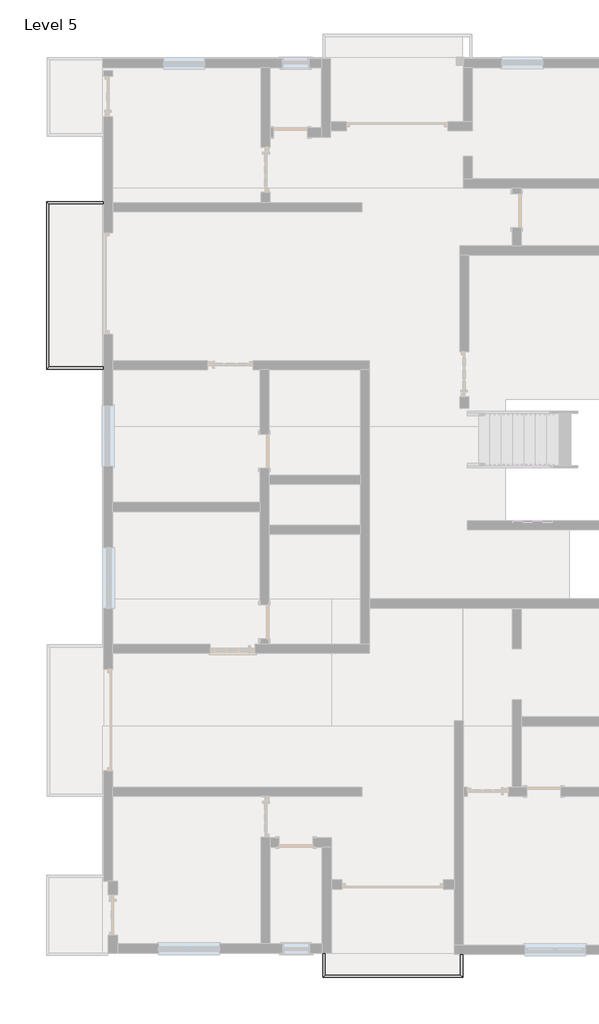
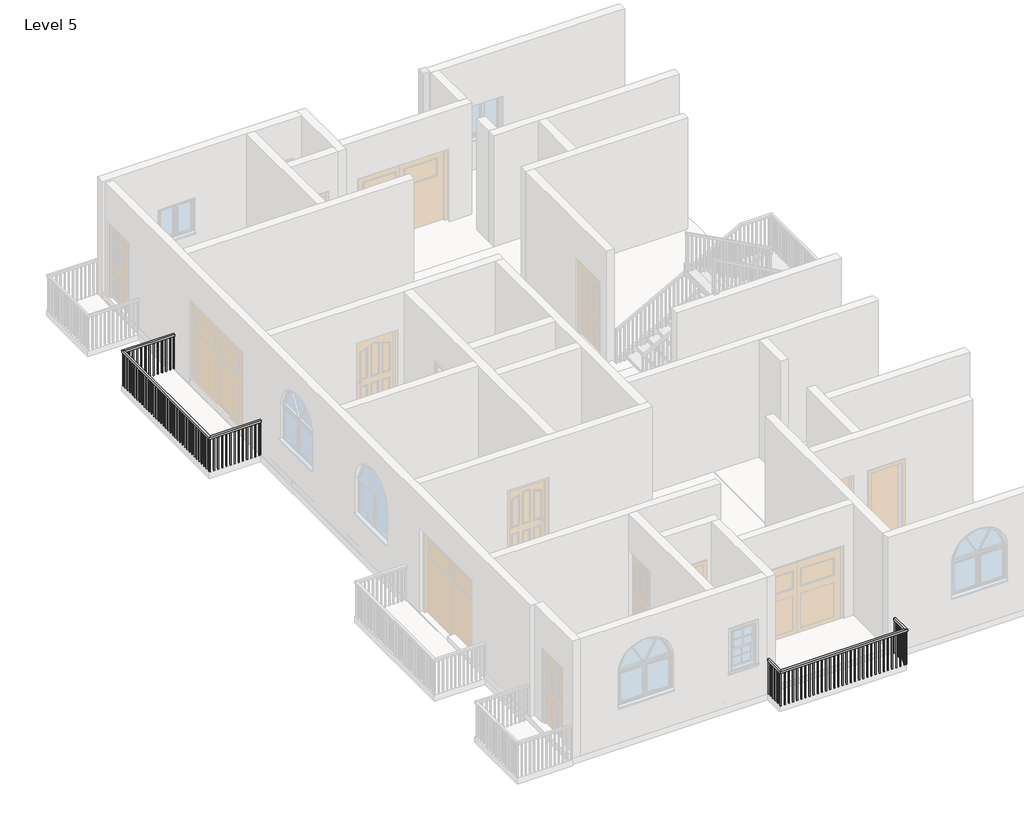
# One storey, part 4 of 7: 2 railings.
"""IFC4 building model written with IfcOpenShell, lengths in millimetres."""

from ifc_helpers import new_model, si_unit, frame, origin, place, context, project, spatial, polyline, outline, extrude, faceted_brep, element, save

model = new_model("IFC4")

# Units and contexts
model_context = context("Model", 3, world=origin())
ifc_project = project(units=[si_unit("LENGTHUNIT", "METRE", prefix="MILLI")], contexts=[model_context])

# Site, building, storey
site = spatial("IfcSite", under=ifc_project)
building = spatial("IfcBuilding", under=site)
storey = spatial("IfcBuildingStorey", under=building, Name="Level 5", Elevation=12192.0)

# Railings
placement = place(None, origin())
element("IfcRailing", 1, ObjectType="Handrail - Rectangular", at=placement, inside=storey, context=model_context, shape_type="SolidModel", body=[
    faceted_brep([(-1375.8109037, -10612.9037749, 13106.4), (-1375.8109037, -10612.9037749, 13055.6), (-1426.6109037, -10612.9037749, 13055.6), (-1426.6109037, -10612.9037749, 13106.4), (-1375.8109037, -11108.2037749, 13106.4), (-1375.8109037, -11108.2037749, 13055.6), (-1426.6109037, -11159.0037749, 13055.6), (-1426.6109037, -11159.0037749, 13106.4), (1659.4890963, -11108.2037749, 13106.4), (1659.4890963, -11108.2037749, 13055.6), (1710.2890963, -11159.0037749, 13055.6), (1710.2890963, -11159.0037749, 13106.4), (1659.4890963, -10638.3037749, 13106.4), (1710.2890963, -10638.3037749, 13106.4), (1710.2890963, -10638.3037749, 13055.6), (1659.4890963, -10638.3037749, 13055.6)], [[[0, 1, 2, 3]], [[1, 0, 4, 5]], [[2, 1, 5, 6]], [[3, 2, 6, 7]], [[0, 3, 7, 4]], [[5, 4, 8, 9]], [[6, 5, 9, 10]], [[7, 6, 10, 11]], [[4, 7, 11, 8]], [[12, 13, 14, 15]], [[9, 8, 12, 15]], [[10, 9, 15, 14]], [[11, 10, 14, 13]], [[8, 11, 13, 12]]]),
    extrude(outline(polyline([(1694.4140963, -10736.7287749), (1675.3640963, -10736.7287749), (1675.3640963, -10717.6787749), (1694.4140963, -10717.6787749), (1694.4140963, -10736.7287749)])), frame((0.0, 0.0, 12192.0), z_axis=(0.0, 0.0, 1.0), x_axis=(1.0, 0.0, 0.0)), (0.0, 0.0, 1.0), 863.6),
    extrude(outline(polyline([(1694.4140963, -10838.3287749), (1675.3640963, -10838.3287749), (1675.3640963, -10819.2787749), (1694.4140963, -10819.2787749), (1694.4140963, -10838.3287749)])), frame((0.0, 0.0, 12192.0), z_axis=(0.0, 0.0, 1.0), x_axis=(1.0, 0.0, 0.0)), (0.0, 0.0, 1.0), 863.6),
    extrude(outline(polyline([(1694.4140963, -10939.9287749), (1675.3640963, -10939.9287749), (1675.3640963, -10920.8787749), (1694.4140963, -10920.8787749), (1694.4140963, -10939.9287749)])), frame((0.0, 0.0, 12192.0), z_axis=(0.0, 0.0, 1.0), x_axis=(1.0, 0.0, 0.0)), (0.0, 0.0, 1.0), 863.6),
    extrude(outline(polyline([(1694.4140963, -11041.5287749), (1675.3640963, -11041.5287749), (1675.3640963, -11022.4787749), (1694.4140963, -11022.4787749), (1694.4140963, -11041.5287749)])), frame((0.0, 0.0, 12192.0), z_axis=(0.0, 0.0, 1.0), x_axis=(1.0, 0.0, 0.0)), (0.0, 0.0, 1.0), 863.6),
    extrude(outline(polyline([(1637.2640963, -11143.1287749), (1637.2640963, -11124.0787749), (1656.3140963, -11124.0787749), (1656.3140963, -11143.1287749), (1637.2640963, -11143.1287749)])), frame((0.0, 0.0, 12192.0), z_axis=(0.0, 0.0, 1.0), x_axis=(1.0, 0.0, 0.0)), (0.0, 0.0, 1.0), 863.6),
    extrude(outline(polyline([(1535.6640963, -11143.1287749), (1535.6640963, -11124.0787749), (1554.7140963, -11124.0787749), (1554.7140963, -11143.1287749), (1535.6640963, -11143.1287749)])), frame((0.0, 0.0, 12192.0), z_axis=(0.0, 0.0, 1.0), x_axis=(1.0, 0.0, 0.0)), (0.0, 0.0, 1.0), 863.6),
    extrude(outline(polyline([(1434.0640963, -11143.1287749), (1434.0640963, -11124.0787749), (1453.1140963, -11124.0787749), (1453.1140963, -11143.1287749), (1434.0640963, -11143.1287749)])), frame((0.0, 0.0, 12192.0), z_axis=(0.0, 0.0, 1.0), x_axis=(1.0, 0.0, 0.0)), (0.0, 0.0, 1.0), 863.6),
    extrude(outline(polyline([(1332.4640963, -11143.1287749), (1332.4640963, -11124.0787749), (1351.5140963, -11124.0787749), (1351.5140963, -11143.1287749), (1332.4640963, -11143.1287749)])), frame((0.0, 0.0, 12192.0), z_axis=(0.0, 0.0, 1.0), x_axis=(1.0, 0.0, 0.0)), (0.0, 0.0, 1.0), 863.6),
    extrude(outline(polyline([(1230.8640963, -11143.1287749), (1230.8640963, -11124.0787749), (1249.9140963, -11124.0787749), (1249.9140963, -11143.1287749), (1230.8640963, -11143.1287749)])), frame((0.0, 0.0, 12192.0), z_axis=(0.0, 0.0, 1.0), x_axis=(1.0, 0.0, 0.0)), (0.0, 0.0, 1.0), 863.6),
    extrude(outline(polyline([(1129.2640963, -11143.1287749), (1129.2640963, -11124.0787749), (1148.3140963, -11124.0787749), (1148.3140963, -11143.1287749), (1129.2640963, -11143.1287749)])), frame((0.0, 0.0, 12192.0), z_axis=(0.0, 0.0, 1.0), x_axis=(1.0, 0.0, 0.0)), (0.0, 0.0, 1.0), 863.6),
    extrude(outline(polyline([(1027.6640963, -11143.1287749), (1027.6640963, -11124.0787749), (1046.7140963, -11124.0787749), (1046.7140963, -11143.1287749), (1027.6640963, -11143.1287749)])), frame((0.0, 0.0, 12192.0), z_axis=(0.0, 0.0, 1.0), x_axis=(1.0, 0.0, 0.0)), (0.0, 0.0, 1.0), 863.6),
    extrude(outline(polyline([(926.0640963, -11143.1287749), (926.0640963, -11124.0787749), (945.1140963, -11124.0787749), (945.1140963, -11143.1287749), (926.0640963, -11143.1287749)])), frame((0.0, 0.0, 12192.0), z_axis=(0.0, 0.0, 1.0), x_axis=(1.0, 0.0, 0.0)), (0.0, 0.0, 1.0), 863.6),
    extrude(outline(polyline([(824.4640963, -11143.1287749), (824.4640963, -11124.0787749), (843.5140963, -11124.0787749), (843.5140963, -11143.1287749), (824.4640963, -11143.1287749)])), frame((0.0, 0.0, 12192.0), z_axis=(0.0, 0.0, 1.0), x_axis=(1.0, 0.0, 0.0)), (0.0, 0.0, 1.0), 863.6),
    extrude(outline(polyline([(722.8640963, -11143.1287749), (722.8640963, -11124.0787749), (741.9140963, -11124.0787749), (741.9140963, -11143.1287749), (722.8640963, -11143.1287749)])), frame((0.0, 0.0, 12192.0), z_axis=(0.0, 0.0, 1.0), x_axis=(1.0, 0.0, 0.0)), (0.0, 0.0, 1.0), 863.6),
    extrude(outline(polyline([(621.2640963, -11143.1287749), (621.2640963, -11124.0787749), (640.3140963, -11124.0787749), (640.3140963, -11143.1287749), (621.2640963, -11143.1287749)])), frame((0.0, 0.0, 12192.0), z_axis=(0.0, 0.0, 1.0), x_axis=(1.0, 0.0, 0.0)), (0.0, 0.0, 1.0), 863.6),
    extrude(outline(polyline([(519.6640963, -11143.1287749), (519.6640963, -11124.0787749), (538.7140963, -11124.0787749), (538.7140963, -11143.1287749), (519.6640963, -11143.1287749)])), frame((0.0, 0.0, 12192.0), z_axis=(0.0, 0.0, 1.0), x_axis=(1.0, 0.0, 0.0)), (0.0, 0.0, 1.0), 863.6),
    extrude(outline(polyline([(418.0640963, -11143.1287749), (418.0640963, -11124.0787749), (437.1140963, -11124.0787749), (437.1140963, -11143.1287749), (418.0640963, -11143.1287749)])), frame((0.0, 0.0, 12192.0), z_axis=(0.0, 0.0, 1.0), x_axis=(1.0, 0.0, 0.0)), (0.0, 0.0, 1.0), 863.6),
    extrude(outline(polyline([(316.4640963, -11143.1287749), (316.4640963, -11124.0787749), (335.5140963, -11124.0787749), (335.5140963, -11143.1287749), (316.4640963, -11143.1287749)])), frame((0.0, 0.0, 12192.0), z_axis=(0.0, 0.0, 1.0), x_axis=(1.0, 0.0, 0.0)), (0.0, 0.0, 1.0), 863.6),
    extrude(outline(polyline([(214.8640963, -11143.1287749), (214.8640963, -11124.0787749), (233.9140963, -11124.0787749), (233.9140963, -11143.1287749), (214.8640963, -11143.1287749)])), frame((0.0, 0.0, 12192.0), z_axis=(0.0, 0.0, 1.0), x_axis=(1.0, 0.0, 0.0)), (0.0, 0.0, 1.0), 863.6),
    extrude(outline(polyline([(113.2640963, -11143.1287749), (113.2640963, -11124.0787749), (132.3140963, -11124.0787749), (132.3140963, -11143.1287749), (113.2640963, -11143.1287749)])), frame((0.0, 0.0, 12192.0), z_axis=(0.0, 0.0, 1.0), x_axis=(1.0, 0.0, 0.0)), (0.0, 0.0, 1.0), 863.6),
    extrude(outline(polyline([(11.6640963, -11143.1287749), (11.6640963, -11124.0787749), (30.7140963, -11124.0787749), (30.7140963, -11143.1287749), (11.6640963, -11143.1287749)])), frame((0.0, 0.0, 12192.0), z_axis=(0.0, 0.0, 1.0), x_axis=(1.0, 0.0, 0.0)), (0.0, 0.0, 1.0), 863.6),
    extrude(outline(polyline([(-89.9359037, -11143.1287749), (-89.9359037, -11124.0787749), (-70.8859037, -11124.0787749), (-70.8859037, -11143.1287749), (-89.9359037, -11143.1287749)])), frame((0.0, 0.0, 12192.0), z_axis=(0.0, 0.0, 1.0), x_axis=(1.0, 0.0, 0.0)), (0.0, 0.0, 1.0), 863.6),
    extrude(outline(polyline([(-191.5359037, -11143.1287749), (-191.5359037, -11124.0787749), (-172.4859037, -11124.0787749), (-172.4859037, -11143.1287749), (-191.5359037, -11143.1287749)])), frame((0.0, 0.0, 12192.0), z_axis=(0.0, 0.0, 1.0), x_axis=(1.0, 0.0, 0.0)), (0.0, 0.0, 1.0), 863.6),
    extrude(outline(polyline([(-293.1359037, -11143.1287749), (-293.1359037, -11124.0787749), (-274.0859037, -11124.0787749), (-274.0859037, -11143.1287749), (-293.1359037, -11143.1287749)])), frame((0.0, 0.0, 12192.0), z_axis=(0.0, 0.0, 1.0), x_axis=(1.0, 0.0, 0.0)), (0.0, 0.0, 1.0), 863.6),
    extrude(outline(polyline([(-394.7359037, -11143.1287749), (-394.7359037, -11124.0787749), (-375.6859037, -11124.0787749), (-375.6859037, -11143.1287749), (-394.7359037, -11143.1287749)])), frame((0.0, 0.0, 12192.0), z_axis=(0.0, 0.0, 1.0), x_axis=(1.0, 0.0, 0.0)), (0.0, 0.0, 1.0), 863.6),
    extrude(outline(polyline([(-496.3359037, -11143.1287749), (-496.3359037, -11124.0787749), (-477.2859037, -11124.0787749), (-477.2859037, -11143.1287749), (-496.3359037, -11143.1287749)])), frame((0.0, 0.0, 12192.0), z_axis=(0.0, 0.0, 1.0), x_axis=(1.0, 0.0, 0.0)), (0.0, 0.0, 1.0), 863.6),
    extrude(outline(polyline([(-597.9359037, -11143.1287749), (-597.9359037, -11124.0787749), (-578.8859037, -11124.0787749), (-578.8859037, -11143.1287749), (-597.9359037, -11143.1287749)])), frame((0.0, 0.0, 12192.0), z_axis=(0.0, 0.0, 1.0), x_axis=(1.0, 0.0, 0.0)), (0.0, 0.0, 1.0), 863.6),
    extrude(outline(polyline([(-699.5359037, -11143.1287749), (-699.5359037, -11124.0787749), (-680.4859037, -11124.0787749), (-680.4859037, -11143.1287749), (-699.5359037, -11143.1287749)])), frame((0.0, 0.0, 12192.0), z_axis=(0.0, 0.0, 1.0), x_axis=(1.0, 0.0, 0.0)), (0.0, 0.0, 1.0), 863.6),
    extrude(outline(polyline([(-801.1359037, -11143.1287749), (-801.1359037, -11124.0787749), (-782.0859037, -11124.0787749), (-782.0859037, -11143.1287749), (-801.1359037, -11143.1287749)])), frame((0.0, 0.0, 12192.0), z_axis=(0.0, 0.0, 1.0), x_axis=(1.0, 0.0, 0.0)), (0.0, 0.0, 1.0), 863.6),
    extrude(outline(polyline([(-902.7359037, -11143.1287749), (-902.7359037, -11124.0787749), (-883.6859037, -11124.0787749), (-883.6859037, -11143.1287749), (-902.7359037, -11143.1287749)])), frame((0.0, 0.0, 12192.0), z_axis=(0.0, 0.0, 1.0), x_axis=(1.0, 0.0, 0.0)), (0.0, 0.0, 1.0), 863.6),
    extrude(outline(polyline([(-1004.3359037, -11143.1287749), (-1004.3359037, -11124.0787749), (-985.2859037, -11124.0787749), (-985.2859037, -11143.1287749), (-1004.3359037, -11143.1287749)])), frame((0.0, 0.0, 12192.0), z_axis=(0.0, 0.0, 1.0), x_axis=(1.0, 0.0, 0.0)), (0.0, 0.0, 1.0), 863.6),
    extrude(outline(polyline([(-1105.9359037, -11143.1287749), (-1105.9359037, -11124.0787749), (-1086.8859037, -11124.0787749), (-1086.8859037, -11143.1287749), (-1105.9359037, -11143.1287749)])), frame((0.0, 0.0, 12192.0), z_axis=(0.0, 0.0, 1.0), x_axis=(1.0, 0.0, 0.0)), (0.0, 0.0, 1.0), 863.6),
    extrude(outline(polyline([(-1207.5359037, -11143.1287749), (-1207.5359037, -11124.0787749), (-1188.4859037, -11124.0787749), (-1188.4859037, -11143.1287749), (-1207.5359037, -11143.1287749)])), frame((0.0, 0.0, 12192.0), z_axis=(0.0, 0.0, 1.0), x_axis=(1.0, 0.0, 0.0)), (0.0, 0.0, 1.0), 863.6),
    extrude(outline(polyline([(-1309.1359037, -11143.1287749), (-1309.1359037, -11124.0787749), (-1290.0859037, -11124.0787749), (-1290.0859037, -11143.1287749), (-1309.1359037, -11143.1287749)])), frame((0.0, 0.0, 12192.0), z_axis=(0.0, 0.0, 1.0), x_axis=(1.0, 0.0, 0.0)), (0.0, 0.0, 1.0), 863.6),
    extrude(outline(polyline([(-1410.7359037, -11111.3787749), (-1391.6859037, -11111.3787749), (-1391.6859037, -11130.4287749), (-1410.7359037, -11130.4287749), (-1410.7359037, -11111.3787749)])), frame((0.0, 0.0, 12192.0), z_axis=(0.0, 0.0, 1.0), x_axis=(1.0, 0.0, 0.0)), (0.0, 0.0, 1.0), 863.6),
    extrude(outline(polyline([(-1410.7359037, -11009.7787749), (-1391.6859037, -11009.7787749), (-1391.6859037, -11028.8287749), (-1410.7359037, -11028.8287749), (-1410.7359037, -11009.7787749)])), frame((0.0, 0.0, 12192.0), z_axis=(0.0, 0.0, 1.0), x_axis=(1.0, 0.0, 0.0)), (0.0, 0.0, 1.0), 863.6),
    extrude(outline(polyline([(-1410.7359037, -10908.1787749), (-1391.6859037, -10908.1787749), (-1391.6859037, -10927.2287749), (-1410.7359037, -10927.2287749), (-1410.7359037, -10908.1787749)])), frame((0.0, 0.0, 12192.0), z_axis=(0.0, 0.0, 1.0), x_axis=(1.0, 0.0, 0.0)), (0.0, 0.0, 1.0), 863.6),
    extrude(outline(polyline([(-1410.7359037, -10806.5787749), (-1391.6859037, -10806.5787749), (-1391.6859037, -10825.6287749), (-1410.7359037, -10825.6287749), (-1410.7359037, -10806.5787749)])), frame((0.0, 0.0, 12192.0), z_axis=(0.0, 0.0, 1.0), x_axis=(1.0, 0.0, 0.0)), (0.0, 0.0, 1.0), 863.6),
    extrude(outline(polyline([(-1410.7359037, -10704.9787749), (-1391.6859037, -10704.9787749), (-1391.6859037, -10724.0287749), (-1410.7359037, -10724.0287749), (-1410.7359037, -10704.9787749)])), frame((0.0, 0.0, 12192.0), z_axis=(0.0, 0.0, 1.0), x_axis=(1.0, 0.0, 0.0)), (0.0, 0.0, 1.0), 863.6),
    extrude(outline(polyline([(1675.3640963, -11143.1287749), (1675.3640963, -11124.0787749), (1694.4140963, -11124.0787749), (1694.4140963, -11143.1287749), (1675.3640963, -11143.1287749)])), frame((0.0, 0.0, 12192.0), z_axis=(0.0, 0.0, 1.0), x_axis=(1.0, 0.0, 0.0)), (0.0, 0.0, 1.0), 863.6),
    extrude(outline(polyline([(-1410.7359037, -11124.0787749), (-1391.6859037, -11124.0787749), (-1391.6859037, -11143.1287749), (-1410.7359037, -11143.1287749), (-1410.7359037, -11124.0787749)])), frame((0.0, 0.0, 12192.0), z_axis=(0.0, 0.0, 1.0), x_axis=(1.0, 0.0, 0.0)), (0.0, 0.0, 1.0), 863.6),
    extrude(outline(polyline([(1694.4140963, -10657.3537749), (1675.3640963, -10657.3537749), (1675.3640963, -10638.3037749), (1694.4140963, -10638.3037749), (1694.4140963, -10657.3537749)])), frame((0.0, 0.0, 12192.0), z_axis=(0.0, 0.0, 1.0), x_axis=(1.0, 0.0, 0.0)), (0.0, 0.0, 1.0), 863.6),
    extrude(outline(polyline([(-1410.7359037, -10612.9037749), (-1391.6859037, -10612.9037749), (-1391.6859037, -10631.9537749), (-1410.7359037, -10631.9537749), (-1410.7359037, -10612.9037749)])), frame((0.0, 0.0, 12192.0), z_axis=(0.0, 0.0, 1.0), x_axis=(1.0, 0.0, 0.0)), (0.0, 0.0, 1.0), 863.6),
])
element("IfcRailing", 2, ObjectType="Handrail - Rectangular", at=placement, inside=storey, context=model_context, shape_type="SolidModel", body=[
    faceted_brep([(-6330.8013636, 6151.0962251, 13106.4), (-6330.8013636, 6151.0962251, 13055.6), (-6330.8013636, 6201.8962251, 13055.6), (-6330.8013636, 6201.8962251, 13106.4), (-7563.8859037, 6151.0962251, 13106.4), (-7563.8859037, 6151.0962251, 13055.6), (-7614.6859037, 6201.8962251, 13055.6), (-7614.6859037, 6201.8962251, 13106.4), (-7563.8859037, 2506.1962251, 13106.4), (-7563.8859037, 2506.1962251, 13055.6), (-7614.6859037, 2455.3962251, 13055.6), (-7614.6859037, 2455.3962251, 13106.4), (-6330.8013636, 2506.1962251, 13106.4), (-6330.8013636, 2455.3962251, 13106.4), (-6330.8013636, 2455.3962251, 13055.6), (-6330.8013636, 2506.1962251, 13055.6)], [[[0, 1, 2, 3]], [[1, 0, 4, 5]], [[2, 1, 5, 6]], [[3, 2, 6, 7]], [[0, 3, 7, 4]], [[5, 4, 8, 9]], [[6, 5, 9, 10]], [[7, 6, 10, 11]], [[4, 7, 11, 8]], [[12, 13, 14, 15]], [[9, 8, 12, 15]], [[10, 9, 15, 14]], [[11, 10, 14, 13]], [[8, 11, 13, 12]]]),
    extrude(outline(polyline([(-6379.6109037, 2471.2712251), (-6379.6109037, 2490.3212251), (-6360.5609037, 2490.3212251), (-6360.5609037, 2471.2712251), (-6379.6109037, 2471.2712251)])), frame((0.0, 0.0, 12192.0), z_axis=(0.0, 0.0, 1.0), x_axis=(1.0, 0.0, 0.0)), (0.0, 0.0, 1.0), 863.6),
    extrude(outline(polyline([(-6481.2109037, 2471.2712251), (-6481.2109037, 2490.3212251), (-6462.1609037, 2490.3212251), (-6462.1609037, 2471.2712251), (-6481.2109037, 2471.2712251)])), frame((0.0, 0.0, 12192.0), z_axis=(0.0, 0.0, 1.0), x_axis=(1.0, 0.0, 0.0)), (0.0, 0.0, 1.0), 863.6),
    extrude(outline(polyline([(-6582.8109037, 2471.2712251), (-6582.8109037, 2490.3212251), (-6563.7609037, 2490.3212251), (-6563.7609037, 2471.2712251), (-6582.8109037, 2471.2712251)])), frame((0.0, 0.0, 12192.0), z_axis=(0.0, 0.0, 1.0), x_axis=(1.0, 0.0, 0.0)), (0.0, 0.0, 1.0), 863.6),
    extrude(outline(polyline([(-6684.4109037, 2471.2712251), (-6684.4109037, 2490.3212251), (-6665.3609037, 2490.3212251), (-6665.3609037, 2471.2712251), (-6684.4109037, 2471.2712251)])), frame((0.0, 0.0, 12192.0), z_axis=(0.0, 0.0, 1.0), x_axis=(1.0, 0.0, 0.0)), (0.0, 0.0, 1.0), 863.6),
    extrude(outline(polyline([(-6786.0109037, 2471.2712251), (-6786.0109037, 2490.3212251), (-6766.9609037, 2490.3212251), (-6766.9609037, 2471.2712251), (-6786.0109037, 2471.2712251)])), frame((0.0, 0.0, 12192.0), z_axis=(0.0, 0.0, 1.0), x_axis=(1.0, 0.0, 0.0)), (0.0, 0.0, 1.0), 863.6),
    extrude(outline(polyline([(-6887.6109037, 2471.2712251), (-6887.6109037, 2490.3212251), (-6868.5609037, 2490.3212251), (-6868.5609037, 2471.2712251), (-6887.6109037, 2471.2712251)])), frame((0.0, 0.0, 12192.0), z_axis=(0.0, 0.0, 1.0), x_axis=(1.0, 0.0, 0.0)), (0.0, 0.0, 1.0), 863.6),
    extrude(outline(polyline([(-6989.2109037, 2471.2712251), (-6989.2109037, 2490.3212251), (-6970.1609037, 2490.3212251), (-6970.1609037, 2471.2712251), (-6989.2109037, 2471.2712251)])), frame((0.0, 0.0, 12192.0), z_axis=(0.0, 0.0, 1.0), x_axis=(1.0, 0.0, 0.0)), (0.0, 0.0, 1.0), 863.6),
    extrude(outline(polyline([(-7090.8109037, 2471.2712251), (-7090.8109037, 2490.3212251), (-7071.7609037, 2490.3212251), (-7071.7609037, 2471.2712251), (-7090.8109037, 2471.2712251)])), frame((0.0, 0.0, 12192.0), z_axis=(0.0, 0.0, 1.0), x_axis=(1.0, 0.0, 0.0)), (0.0, 0.0, 1.0), 863.6),
    extrude(outline(polyline([(-7192.4109037, 2471.2712251), (-7192.4109037, 2490.3212251), (-7173.3609037, 2490.3212251), (-7173.3609037, 2471.2712251), (-7192.4109037, 2471.2712251)])), frame((0.0, 0.0, 12192.0), z_axis=(0.0, 0.0, 1.0), x_axis=(1.0, 0.0, 0.0)), (0.0, 0.0, 1.0), 863.6),
    extrude(outline(polyline([(-7294.0109037, 2471.2712251), (-7294.0109037, 2490.3212251), (-7274.9609037, 2490.3212251), (-7274.9609037, 2471.2712251), (-7294.0109037, 2471.2712251)])), frame((0.0, 0.0, 12192.0), z_axis=(0.0, 0.0, 1.0), x_axis=(1.0, 0.0, 0.0)), (0.0, 0.0, 1.0), 863.6),
    extrude(outline(polyline([(-7395.6109037, 2471.2712251), (-7395.6109037, 2490.3212251), (-7376.5609037, 2490.3212251), (-7376.5609037, 2471.2712251), (-7395.6109037, 2471.2712251)])), frame((0.0, 0.0, 12192.0), z_axis=(0.0, 0.0, 1.0), x_axis=(1.0, 0.0, 0.0)), (0.0, 0.0, 1.0), 863.6),
    extrude(outline(polyline([(-7497.2109037, 2471.2712251), (-7497.2109037, 2490.3212251), (-7478.1609037, 2490.3212251), (-7478.1609037, 2471.2712251), (-7497.2109037, 2471.2712251)])), frame((0.0, 0.0, 12192.0), z_axis=(0.0, 0.0, 1.0), x_axis=(1.0, 0.0, 0.0)), (0.0, 0.0, 1.0), 863.6),
    extrude(outline(polyline([(-7598.8109037, 2528.4212251), (-7579.7609037, 2528.4212251), (-7579.7609037, 2509.3712251), (-7598.8109037, 2509.3712251), (-7598.8109037, 2528.4212251)])), frame((0.0, 0.0, 12192.0), z_axis=(0.0, 0.0, 1.0), x_axis=(1.0, 0.0, 0.0)), (0.0, 0.0, 1.0), 863.6),
    extrude(outline(polyline([(-7598.8109037, 2630.0212251), (-7579.7609037, 2630.0212251), (-7579.7609037, 2610.9712251), (-7598.8109037, 2610.9712251), (-7598.8109037, 2630.0212251)])), frame((0.0, 0.0, 12192.0), z_axis=(0.0, 0.0, 1.0), x_axis=(1.0, 0.0, 0.0)), (0.0, 0.0, 1.0), 863.6),
    extrude(outline(polyline([(-7598.8109037, 2731.6212251), (-7579.7609037, 2731.6212251), (-7579.7609037, 2712.5712251), (-7598.8109037, 2712.5712251), (-7598.8109037, 2731.6212251)])), frame((0.0, 0.0, 12192.0), z_axis=(0.0, 0.0, 1.0), x_axis=(1.0, 0.0, 0.0)), (0.0, 0.0, 1.0), 863.6),
    extrude(outline(polyline([(-7598.8109037, 2833.2212251), (-7579.7609037, 2833.2212251), (-7579.7609037, 2814.1712251), (-7598.8109037, 2814.1712251), (-7598.8109037, 2833.2212251)])), frame((0.0, 0.0, 12192.0), z_axis=(0.0, 0.0, 1.0), x_axis=(1.0, 0.0, 0.0)), (0.0, 0.0, 1.0), 863.6),
    extrude(outline(polyline([(-7598.8109037, 2934.8212251), (-7579.7609037, 2934.8212251), (-7579.7609037, 2915.7712251), (-7598.8109037, 2915.7712251), (-7598.8109037, 2934.8212251)])), frame((0.0, 0.0, 12192.0), z_axis=(0.0, 0.0, 1.0), x_axis=(1.0, 0.0, 0.0)), (0.0, 0.0, 1.0), 863.6),
    extrude(outline(polyline([(-7598.8109037, 3036.4212251), (-7579.7609037, 3036.4212251), (-7579.7609037, 3017.3712251), (-7598.8109037, 3017.3712251), (-7598.8109037, 3036.4212251)])), frame((0.0, 0.0, 12192.0), z_axis=(0.0, 0.0, 1.0), x_axis=(1.0, 0.0, 0.0)), (0.0, 0.0, 1.0), 863.6),
    extrude(outline(polyline([(-7598.8109037, 3138.0212251), (-7579.7609037, 3138.0212251), (-7579.7609037, 3118.9712251), (-7598.8109037, 3118.9712251), (-7598.8109037, 3138.0212251)])), frame((0.0, 0.0, 12192.0), z_axis=(0.0, 0.0, 1.0), x_axis=(1.0, 0.0, 0.0)), (0.0, 0.0, 1.0), 863.6),
    extrude(outline(polyline([(-7598.8109037, 3239.6212251), (-7579.7609037, 3239.6212251), (-7579.7609037, 3220.5712251), (-7598.8109037, 3220.5712251), (-7598.8109037, 3239.6212251)])), frame((0.0, 0.0, 12192.0), z_axis=(0.0, 0.0, 1.0), x_axis=(1.0, 0.0, 0.0)), (0.0, 0.0, 1.0), 863.6),
    extrude(outline(polyline([(-7598.8109037, 3341.2212251), (-7579.7609037, 3341.2212251), (-7579.7609037, 3322.1712251), (-7598.8109037, 3322.1712251), (-7598.8109037, 3341.2212251)])), frame((0.0, 0.0, 12192.0), z_axis=(0.0, 0.0, 1.0), x_axis=(1.0, 0.0, 0.0)), (0.0, 0.0, 1.0), 863.6),
    extrude(outline(polyline([(-7598.8109037, 3442.8212251), (-7579.7609037, 3442.8212251), (-7579.7609037, 3423.7712251), (-7598.8109037, 3423.7712251), (-7598.8109037, 3442.8212251)])), frame((0.0, 0.0, 12192.0), z_axis=(0.0, 0.0, 1.0), x_axis=(1.0, 0.0, 0.0)), (0.0, 0.0, 1.0), 863.6),
    extrude(outline(polyline([(-7598.8109037, 3544.4212251), (-7579.7609037, 3544.4212251), (-7579.7609037, 3525.3712251), (-7598.8109037, 3525.3712251), (-7598.8109037, 3544.4212251)])), frame((0.0, 0.0, 12192.0), z_axis=(0.0, 0.0, 1.0), x_axis=(1.0, 0.0, 0.0)), (0.0, 0.0, 1.0), 863.6),
    extrude(outline(polyline([(-7598.8109037, 3646.0212251), (-7579.7609037, 3646.0212251), (-7579.7609037, 3626.9712251), (-7598.8109037, 3626.9712251), (-7598.8109037, 3646.0212251)])), frame((0.0, 0.0, 12192.0), z_axis=(0.0, 0.0, 1.0), x_axis=(1.0, 0.0, 0.0)), (0.0, 0.0, 1.0), 863.6),
    extrude(outline(polyline([(-7598.8109037, 3747.6212251), (-7579.7609037, 3747.6212251), (-7579.7609037, 3728.5712251), (-7598.8109037, 3728.5712251), (-7598.8109037, 3747.6212251)])), frame((0.0, 0.0, 12192.0), z_axis=(0.0, 0.0, 1.0), x_axis=(1.0, 0.0, 0.0)), (0.0, 0.0, 1.0), 863.6),
    extrude(outline(polyline([(-7598.8109037, 3849.2212251), (-7579.7609037, 3849.2212251), (-7579.7609037, 3830.1712251), (-7598.8109037, 3830.1712251), (-7598.8109037, 3849.2212251)])), frame((0.0, 0.0, 12192.0), z_axis=(0.0, 0.0, 1.0), x_axis=(1.0, 0.0, 0.0)), (0.0, 0.0, 1.0), 863.6),
    extrude(outline(polyline([(-7598.8109037, 3950.8212251), (-7579.7609037, 3950.8212251), (-7579.7609037, 3931.7712251), (-7598.8109037, 3931.7712251), (-7598.8109037, 3950.8212251)])), frame((0.0, 0.0, 12192.0), z_axis=(0.0, 0.0, 1.0), x_axis=(1.0, 0.0, 0.0)), (0.0, 0.0, 1.0), 863.6),
    extrude(outline(polyline([(-7598.8109037, 4052.4212251), (-7579.7609037, 4052.4212251), (-7579.7609037, 4033.3712251), (-7598.8109037, 4033.3712251), (-7598.8109037, 4052.4212251)])), frame((0.0, 0.0, 12192.0), z_axis=(0.0, 0.0, 1.0), x_axis=(1.0, 0.0, 0.0)), (0.0, 0.0, 1.0), 863.6),
    extrude(outline(polyline([(-7598.8109037, 4154.0212251), (-7579.7609037, 4154.0212251), (-7579.7609037, 4134.9712251), (-7598.8109037, 4134.9712251), (-7598.8109037, 4154.0212251)])), frame((0.0, 0.0, 12192.0), z_axis=(0.0, 0.0, 1.0), x_axis=(1.0, 0.0, 0.0)), (0.0, 0.0, 1.0), 863.6),
    extrude(outline(polyline([(-7598.8109037, 4255.6212251), (-7579.7609037, 4255.6212251), (-7579.7609037, 4236.5712251), (-7598.8109037, 4236.5712251), (-7598.8109037, 4255.6212251)])), frame((0.0, 0.0, 12192.0), z_axis=(0.0, 0.0, 1.0), x_axis=(1.0, 0.0, 0.0)), (0.0, 0.0, 1.0), 863.6),
    extrude(outline(polyline([(-7598.8109037, 4357.2212251), (-7579.7609037, 4357.2212251), (-7579.7609037, 4338.1712251), (-7598.8109037, 4338.1712251), (-7598.8109037, 4357.2212251)])), frame((0.0, 0.0, 12192.0), z_axis=(0.0, 0.0, 1.0), x_axis=(1.0, 0.0, 0.0)), (0.0, 0.0, 1.0), 863.6),
    extrude(outline(polyline([(-7598.8109037, 4458.8212251), (-7579.7609037, 4458.8212251), (-7579.7609037, 4439.7712251), (-7598.8109037, 4439.7712251), (-7598.8109037, 4458.8212251)])), frame((0.0, 0.0, 12192.0), z_axis=(0.0, 0.0, 1.0), x_axis=(1.0, 0.0, 0.0)), (0.0, 0.0, 1.0), 863.6),
    extrude(outline(polyline([(-7598.8109037, 4560.4212251), (-7579.7609037, 4560.4212251), (-7579.7609037, 4541.3712251), (-7598.8109037, 4541.3712251), (-7598.8109037, 4560.4212251)])), frame((0.0, 0.0, 12192.0), z_axis=(0.0, 0.0, 1.0), x_axis=(1.0, 0.0, 0.0)), (0.0, 0.0, 1.0), 863.6),
    extrude(outline(polyline([(-7598.8109037, 4662.0212251), (-7579.7609037, 4662.0212251), (-7579.7609037, 4642.9712251), (-7598.8109037, 4642.9712251), (-7598.8109037, 4662.0212251)])), frame((0.0, 0.0, 12192.0), z_axis=(0.0, 0.0, 1.0), x_axis=(1.0, 0.0, 0.0)), (0.0, 0.0, 1.0), 863.6),
    extrude(outline(polyline([(-7598.8109037, 4763.6212251), (-7579.7609037, 4763.6212251), (-7579.7609037, 4744.5712251), (-7598.8109037, 4744.5712251), (-7598.8109037, 4763.6212251)])), frame((0.0, 0.0, 12192.0), z_axis=(0.0, 0.0, 1.0), x_axis=(1.0, 0.0, 0.0)), (0.0, 0.0, 1.0), 863.6),
    extrude(outline(polyline([(-7598.8109037, 4865.2212251), (-7579.7609037, 4865.2212251), (-7579.7609037, 4846.1712251), (-7598.8109037, 4846.1712251), (-7598.8109037, 4865.2212251)])), frame((0.0, 0.0, 12192.0), z_axis=(0.0, 0.0, 1.0), x_axis=(1.0, 0.0, 0.0)), (0.0, 0.0, 1.0), 863.6),
    extrude(outline(polyline([(-7598.8109037, 4966.8212251), (-7579.7609037, 4966.8212251), (-7579.7609037, 4947.7712251), (-7598.8109037, 4947.7712251), (-7598.8109037, 4966.8212251)])), frame((0.0, 0.0, 12192.0), z_axis=(0.0, 0.0, 1.0), x_axis=(1.0, 0.0, 0.0)), (0.0, 0.0, 1.0), 863.6),
    extrude(outline(polyline([(-7598.8109037, 5068.4212251), (-7579.7609037, 5068.4212251), (-7579.7609037, 5049.3712251), (-7598.8109037, 5049.3712251), (-7598.8109037, 5068.4212251)])), frame((0.0, 0.0, 12192.0), z_axis=(0.0, 0.0, 1.0), x_axis=(1.0, 0.0, 0.0)), (0.0, 0.0, 1.0), 863.6),
    extrude(outline(polyline([(-7598.8109037, 5170.0212251), (-7579.7609037, 5170.0212251), (-7579.7609037, 5150.9712251), (-7598.8109037, 5150.9712251), (-7598.8109037, 5170.0212251)])), frame((0.0, 0.0, 12192.0), z_axis=(0.0, 0.0, 1.0), x_axis=(1.0, 0.0, 0.0)), (0.0, 0.0, 1.0), 863.6),
    extrude(outline(polyline([(-7598.8109037, 5271.6212251), (-7579.7609037, 5271.6212251), (-7579.7609037, 5252.5712251), (-7598.8109037, 5252.5712251), (-7598.8109037, 5271.6212251)])), frame((0.0, 0.0, 12192.0), z_axis=(0.0, 0.0, 1.0), x_axis=(1.0, 0.0, 0.0)), (0.0, 0.0, 1.0), 863.6),
    extrude(outline(polyline([(-7598.8109037, 5373.2212251), (-7579.7609037, 5373.2212251), (-7579.7609037, 5354.1712251), (-7598.8109037, 5354.1712251), (-7598.8109037, 5373.2212251)])), frame((0.0, 0.0, 12192.0), z_axis=(0.0, 0.0, 1.0), x_axis=(1.0, 0.0, 0.0)), (0.0, 0.0, 1.0), 863.6),
    extrude(outline(polyline([(-7598.8109037, 5474.8212251), (-7579.7609037, 5474.8212251), (-7579.7609037, 5455.7712251), (-7598.8109037, 5455.7712251), (-7598.8109037, 5474.8212251)])), frame((0.0, 0.0, 12192.0), z_axis=(0.0, 0.0, 1.0), x_axis=(1.0, 0.0, 0.0)), (0.0, 0.0, 1.0), 863.6),
    extrude(outline(polyline([(-7598.8109037, 5576.4212251), (-7579.7609037, 5576.4212251), (-7579.7609037, 5557.3712251), (-7598.8109037, 5557.3712251), (-7598.8109037, 5576.4212251)])), frame((0.0, 0.0, 12192.0), z_axis=(0.0, 0.0, 1.0), x_axis=(1.0, 0.0, 0.0)), (0.0, 0.0, 1.0), 863.6),
    extrude(outline(polyline([(-7598.8109037, 5678.0212251), (-7579.7609037, 5678.0212251), (-7579.7609037, 5658.9712251), (-7598.8109037, 5658.9712251), (-7598.8109037, 5678.0212251)])), frame((0.0, 0.0, 12192.0), z_axis=(0.0, 0.0, 1.0), x_axis=(1.0, 0.0, 0.0)), (0.0, 0.0, 1.0), 863.6),
    extrude(outline(polyline([(-7598.8109037, 5779.6212251), (-7579.7609037, 5779.6212251), (-7579.7609037, 5760.5712251), (-7598.8109037, 5760.5712251), (-7598.8109037, 5779.6212251)])), frame((0.0, 0.0, 12192.0), z_axis=(0.0, 0.0, 1.0), x_axis=(1.0, 0.0, 0.0)), (0.0, 0.0, 1.0), 863.6),
    extrude(outline(polyline([(-7598.8109037, 5881.2212251), (-7579.7609037, 5881.2212251), (-7579.7609037, 5862.1712251), (-7598.8109037, 5862.1712251), (-7598.8109037, 5881.2212251)])), frame((0.0, 0.0, 12192.0), z_axis=(0.0, 0.0, 1.0), x_axis=(1.0, 0.0, 0.0)), (0.0, 0.0, 1.0), 863.6),
    extrude(outline(polyline([(-7598.8109037, 5982.8212251), (-7579.7609037, 5982.8212251), (-7579.7609037, 5963.7712251), (-7598.8109037, 5963.7712251), (-7598.8109037, 5982.8212251)])), frame((0.0, 0.0, 12192.0), z_axis=(0.0, 0.0, 1.0), x_axis=(1.0, 0.0, 0.0)), (0.0, 0.0, 1.0), 863.6),
    extrude(outline(polyline([(-7598.8109037, 6084.4212251), (-7579.7609037, 6084.4212251), (-7579.7609037, 6065.3712251), (-7598.8109037, 6065.3712251), (-7598.8109037, 6084.4212251)])), frame((0.0, 0.0, 12192.0), z_axis=(0.0, 0.0, 1.0), x_axis=(1.0, 0.0, 0.0)), (0.0, 0.0, 1.0), 863.6),
    extrude(outline(polyline([(-7540.4763636, 6186.0212251), (-7540.4763636, 6166.9712251), (-7559.5263636, 6166.9712251), (-7559.5263636, 6186.0212251), (-7540.4763636, 6186.0212251)])), frame((0.0, 0.0, 12192.0), z_axis=(0.0, 0.0, 1.0), x_axis=(1.0, 0.0, 0.0)), (0.0, 0.0, 1.0), 863.6),
    extrude(outline(polyline([(-7438.8763636, 6186.0212251), (-7438.8763636, 6166.9712251), (-7457.9263636, 6166.9712251), (-7457.9263636, 6186.0212251), (-7438.8763636, 6186.0212251)])), frame((0.0, 0.0, 12192.0), z_axis=(0.0, 0.0, 1.0), x_axis=(1.0, 0.0, 0.0)), (0.0, 0.0, 1.0), 863.6),
    extrude(outline(polyline([(-7337.2763636, 6186.0212251), (-7337.2763636, 6166.9712251), (-7356.3263636, 6166.9712251), (-7356.3263636, 6186.0212251), (-7337.2763636, 6186.0212251)])), frame((0.0, 0.0, 12192.0), z_axis=(0.0, 0.0, 1.0), x_axis=(1.0, 0.0, 0.0)), (0.0, 0.0, 1.0), 863.6),
    extrude(outline(polyline([(-7235.6763636, 6186.0212251), (-7235.6763636, 6166.9712251), (-7254.7263636, 6166.9712251), (-7254.7263636, 6186.0212251), (-7235.6763636, 6186.0212251)])), frame((0.0, 0.0, 12192.0), z_axis=(0.0, 0.0, 1.0), x_axis=(1.0, 0.0, 0.0)), (0.0, 0.0, 1.0), 863.6),
    extrude(outline(polyline([(-7134.0763636, 6186.0212251), (-7134.0763636, 6166.9712251), (-7153.1263636, 6166.9712251), (-7153.1263636, 6186.0212251), (-7134.0763636, 6186.0212251)])), frame((0.0, 0.0, 12192.0), z_axis=(0.0, 0.0, 1.0), x_axis=(1.0, 0.0, 0.0)), (0.0, 0.0, 1.0), 863.6),
    extrude(outline(polyline([(-7032.4763636, 6186.0212251), (-7032.4763636, 6166.9712251), (-7051.5263636, 6166.9712251), (-7051.5263636, 6186.0212251), (-7032.4763636, 6186.0212251)])), frame((0.0, 0.0, 12192.0), z_axis=(0.0, 0.0, 1.0), x_axis=(1.0, 0.0, 0.0)), (0.0, 0.0, 1.0), 863.6),
    extrude(outline(polyline([(-6930.8763636, 6186.0212251), (-6930.8763636, 6166.9712251), (-6949.9263636, 6166.9712251), (-6949.9263636, 6186.0212251), (-6930.8763636, 6186.0212251)])), frame((0.0, 0.0, 12192.0), z_axis=(0.0, 0.0, 1.0), x_axis=(1.0, 0.0, 0.0)), (0.0, 0.0, 1.0), 863.6),
    extrude(outline(polyline([(-6829.2763636, 6186.0212251), (-6829.2763636, 6166.9712251), (-6848.3263636, 6166.9712251), (-6848.3263636, 6186.0212251), (-6829.2763636, 6186.0212251)])), frame((0.0, 0.0, 12192.0), z_axis=(0.0, 0.0, 1.0), x_axis=(1.0, 0.0, 0.0)), (0.0, 0.0, 1.0), 863.6),
    extrude(outline(polyline([(-6727.6763636, 6186.0212251), (-6727.6763636, 6166.9712251), (-6746.7263636, 6166.9712251), (-6746.7263636, 6186.0212251), (-6727.6763636, 6186.0212251)])), frame((0.0, 0.0, 12192.0), z_axis=(0.0, 0.0, 1.0), x_axis=(1.0, 0.0, 0.0)), (0.0, 0.0, 1.0), 863.6),
    extrude(outline(polyline([(-6626.0763636, 6186.0212251), (-6626.0763636, 6166.9712251), (-6645.1263636, 6166.9712251), (-6645.1263636, 6186.0212251), (-6626.0763636, 6186.0212251)])), frame((0.0, 0.0, 12192.0), z_axis=(0.0, 0.0, 1.0), x_axis=(1.0, 0.0, 0.0)), (0.0, 0.0, 1.0), 863.6),
    extrude(outline(polyline([(-6524.4763636, 6186.0212251), (-6524.4763636, 6166.9712251), (-6543.5263636, 6166.9712251), (-6543.5263636, 6186.0212251), (-6524.4763636, 6186.0212251)])), frame((0.0, 0.0, 12192.0), z_axis=(0.0, 0.0, 1.0), x_axis=(1.0, 0.0, 0.0)), (0.0, 0.0, 1.0), 863.6),
    extrude(outline(polyline([(-6422.8763636, 6186.0212251), (-6422.8763636, 6166.9712251), (-6441.9263636, 6166.9712251), (-6441.9263636, 6186.0212251), (-6422.8763636, 6186.0212251)])), frame((0.0, 0.0, 12192.0), z_axis=(0.0, 0.0, 1.0), x_axis=(1.0, 0.0, 0.0)), (0.0, 0.0, 1.0), 863.6),
    extrude(outline(polyline([(-7598.8109037, 2490.3212251), (-7579.7609037, 2490.3212251), (-7579.7609037, 2471.2712251), (-7598.8109037, 2471.2712251), (-7598.8109037, 2490.3212251)])), frame((0.0, 0.0, 12192.0), z_axis=(0.0, 0.0, 1.0), x_axis=(1.0, 0.0, 0.0)), (0.0, 0.0, 1.0), 863.6),
    extrude(outline(polyline([(-7579.7609037, 6186.0212251), (-7579.7609037, 6166.9712251), (-7598.8109037, 6166.9712251), (-7598.8109037, 6186.0212251), (-7579.7609037, 6186.0212251)])), frame((0.0, 0.0, 12192.0), z_axis=(0.0, 0.0, 1.0), x_axis=(1.0, 0.0, 0.0)), (0.0, 0.0, 1.0), 863.6),
    extrude(outline(polyline([(-6349.8513636, 2471.2712251), (-6349.8513636, 2490.3212251), (-6330.8013636, 2490.3212251), (-6330.8013636, 2471.2712251), (-6349.8513636, 2471.2712251)])), frame((0.0, 0.0, 12192.0), z_axis=(0.0, 0.0, 1.0), x_axis=(1.0, 0.0, 0.0)), (0.0, 0.0, 1.0), 863.6),
    extrude(outline(polyline([(-6330.8013636, 6186.0212251), (-6330.8013636, 6166.9712251), (-6349.8513636, 6166.9712251), (-6349.8513636, 6186.0212251), (-6330.8013636, 6186.0212251)])), frame((0.0, 0.0, 12192.0), z_axis=(0.0, 0.0, 1.0), x_axis=(1.0, 0.0, 0.0)), (0.0, 0.0, 1.0), 863.6),
])

save(model, "model.ifc")

# Revit data of these elements
# Type "Handrail - Rectangular"
#   Assembly Code = "C2010400"
#   built-in parameter 1008612 = 0.0416667 (stored number, unit not read)
#   built-in parameter 1008611 = 0.0416667 (stored number, unit not read)
#   built-in parameter 1008609 = 0.333333 (stored number, unit not read)
#   built-in parameter 1008604 = 0.166667 (stored number, unit not read)
#   built-in parameter 1008603 = 0.166667 (stored number, unit not read)
#   Railing Height = 3' - 0"
#   built-in parameter 1008630 = 2
#   built-in parameter 1008610 = 2
#   built-in parameter 1008618 = Baluster - Square : 3/4"
# Elements 1, 2 (IfcRailing, "Handrail - Rectangular")
#   Phase Created = New Construction
